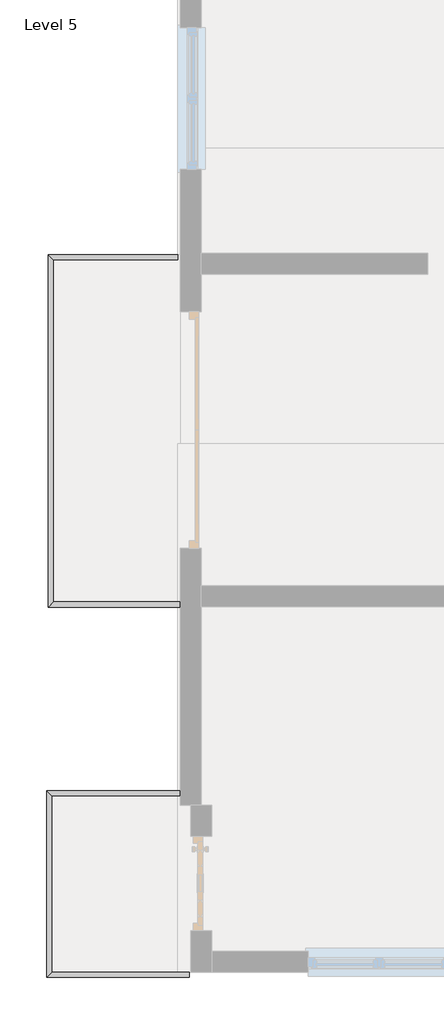
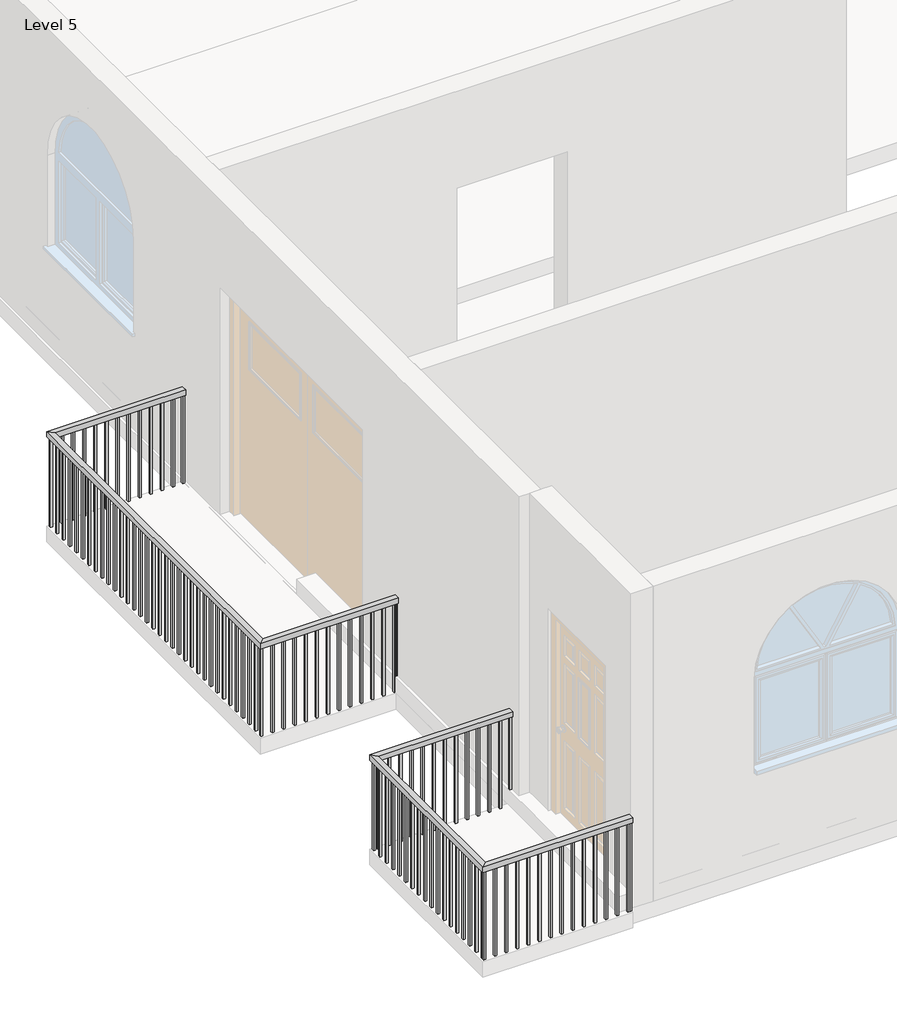
# One storey, part 3 of 7: 2 railings.
"""IFC4 building model written with IfcOpenShell, lengths in millimetres."""

from ifc_helpers import new_model, si_unit, frame, origin, place, context, project, spatial, polyline, outline, extrude, faceted_brep, element, save

model = new_model("IFC4")

# Units and contexts
model_context = context("Model", 3, world=origin())
ifc_project = project(units=[si_unit("LENGTHUNIT", "METRE", prefix="MILLI")], contexts=[model_context])

# Site, building, storey
site = spatial("IfcSite", under=ifc_project)
building = spatial("IfcBuilding", under=site)
storey = spatial("IfcBuildingStorey", under=building, Name="Level 5", Elevation=12192.0)

# Railings
placement = place(None, origin())
element("IfcRailing", 1, ObjectType="Handrail - Rectangular", at=placement, inside=storey, context=model_context, shape_type="SolidModel", body=[
    faceted_brep([(-6354.2109037, -3767.6037749, 13106.4), (-6354.2109037, -3767.6037749, 13055.6), (-6354.2109037, -3716.8037749, 13055.6), (-6354.2109037, -3716.8037749, 13106.4), (-7548.0109037, -3767.6037749, 13106.4), (-7548.0109037, -3767.6037749, 13055.6), (-7598.8109037, -3716.8037749, 13055.6), (-7598.8109037, -3716.8037749, 13106.4), (-7548.0109037, -7054.4894702, 13106.4), (-7548.0109037, -7054.4894702, 13055.6), (-7598.8109037, -7105.2894702, 13055.6), (-7598.8109037, -7105.2894702, 13106.4), (-6330.8013636, -7054.4894702, 13106.4), (-6330.8013636, -7105.2894702, 13106.4), (-6330.8013636, -7105.2894702, 13055.6), (-6330.8013636, -7054.4894702, 13055.6)], [[[0, 1, 2, 3]], [[1, 0, 4, 5]], [[2, 1, 5, 6]], [[3, 2, 6, 7]], [[0, 3, 7, 4]], [[5, 4, 8, 9]], [[6, 5, 9, 10]], [[7, 6, 10, 11]], [[4, 7, 11, 8]], [[12, 13, 14, 15]], [[9, 8, 12, 15]], [[10, 9, 15, 14]], [[11, 10, 14, 13]], [[8, 11, 13, 12]]]),
    extrude(outline(polyline([(-6363.7359037, -7089.4144702), (-6363.7359037, -7070.3644702), (-6344.6859037, -7070.3644702), (-6344.6859037, -7089.4144702), (-6363.7359037, -7089.4144702)])), frame((0.0, 0.0, 12192.0), z_axis=(0.0, 0.0, 1.0), x_axis=(1.0, 0.0, 0.0)), (0.0, 0.0, 1.0), 863.6),
    extrude(outline(polyline([(-6465.3359037, -7089.4144702), (-6465.3359037, -7070.3644702), (-6446.2859037, -7070.3644702), (-6446.2859037, -7089.4144702), (-6465.3359037, -7089.4144702)])), frame((0.0, 0.0, 12192.0), z_axis=(0.0, 0.0, 1.0), x_axis=(1.0, 0.0, 0.0)), (0.0, 0.0, 1.0), 863.6),
    extrude(outline(polyline([(-6566.9359037, -7089.4144702), (-6566.9359037, -7070.3644702), (-6547.8859037, -7070.3644702), (-6547.8859037, -7089.4144702), (-6566.9359037, -7089.4144702)])), frame((0.0, 0.0, 12192.0), z_axis=(0.0, 0.0, 1.0), x_axis=(1.0, 0.0, 0.0)), (0.0, 0.0, 1.0), 863.6),
    extrude(outline(polyline([(-6668.5359037, -7089.4144702), (-6668.5359037, -7070.3644702), (-6649.4859037, -7070.3644702), (-6649.4859037, -7089.4144702), (-6668.5359037, -7089.4144702)])), frame((0.0, 0.0, 12192.0), z_axis=(0.0, 0.0, 1.0), x_axis=(1.0, 0.0, 0.0)), (0.0, 0.0, 1.0), 863.6),
    extrude(outline(polyline([(-6770.1359037, -7089.4144702), (-6770.1359037, -7070.3644702), (-6751.0859037, -7070.3644702), (-6751.0859037, -7089.4144702), (-6770.1359037, -7089.4144702)])), frame((0.0, 0.0, 12192.0), z_axis=(0.0, 0.0, 1.0), x_axis=(1.0, 0.0, 0.0)), (0.0, 0.0, 1.0), 863.6),
    extrude(outline(polyline([(-6871.7359037, -7089.4144702), (-6871.7359037, -7070.3644702), (-6852.6859037, -7070.3644702), (-6852.6859037, -7089.4144702), (-6871.7359037, -7089.4144702)])), frame((0.0, 0.0, 12192.0), z_axis=(0.0, 0.0, 1.0), x_axis=(1.0, 0.0, 0.0)), (0.0, 0.0, 1.0), 863.6),
    extrude(outline(polyline([(-6973.3359037, -7089.4144702), (-6973.3359037, -7070.3644702), (-6954.2859037, -7070.3644702), (-6954.2859037, -7089.4144702), (-6973.3359037, -7089.4144702)])), frame((0.0, 0.0, 12192.0), z_axis=(0.0, 0.0, 1.0), x_axis=(1.0, 0.0, 0.0)), (0.0, 0.0, 1.0), 863.6),
    extrude(outline(polyline([(-7074.9359037, -7089.4144702), (-7074.9359037, -7070.3644702), (-7055.8859037, -7070.3644702), (-7055.8859037, -7089.4144702), (-7074.9359037, -7089.4144702)])), frame((0.0, 0.0, 12192.0), z_axis=(0.0, 0.0, 1.0), x_axis=(1.0, 0.0, 0.0)), (0.0, 0.0, 1.0), 863.6),
    extrude(outline(polyline([(-7176.5359037, -7089.4144702), (-7176.5359037, -7070.3644702), (-7157.4859037, -7070.3644702), (-7157.4859037, -7089.4144702), (-7176.5359037, -7089.4144702)])), frame((0.0, 0.0, 12192.0), z_axis=(0.0, 0.0, 1.0), x_axis=(1.0, 0.0, 0.0)), (0.0, 0.0, 1.0), 863.6),
    extrude(outline(polyline([(-7278.1359037, -7089.4144702), (-7278.1359037, -7070.3644702), (-7259.0859037, -7070.3644702), (-7259.0859037, -7089.4144702), (-7278.1359037, -7089.4144702)])), frame((0.0, 0.0, 12192.0), z_axis=(0.0, 0.0, 1.0), x_axis=(1.0, 0.0, 0.0)), (0.0, 0.0, 1.0), 863.6),
    extrude(outline(polyline([(-7379.7359037, -7089.4144702), (-7379.7359037, -7070.3644702), (-7360.6859037, -7070.3644702), (-7360.6859037, -7089.4144702), (-7379.7359037, -7089.4144702)])), frame((0.0, 0.0, 12192.0), z_axis=(0.0, 0.0, 1.0), x_axis=(1.0, 0.0, 0.0)), (0.0, 0.0, 1.0), 863.6),
    extrude(outline(polyline([(-7481.3359037, -7089.4144702), (-7481.3359037, -7070.3644702), (-7462.2859037, -7070.3644702), (-7462.2859037, -7089.4144702), (-7481.3359037, -7089.4144702)])), frame((0.0, 0.0, 12192.0), z_axis=(0.0, 0.0, 1.0), x_axis=(1.0, 0.0, 0.0)), (0.0, 0.0, 1.0), 863.6),
    extrude(outline(polyline([(-7582.9359037, -6983.8787749), (-7563.8859037, -6983.8787749), (-7563.8859037, -7002.9287749), (-7582.9359037, -7002.9287749), (-7582.9359037, -6983.8787749)])), frame((0.0, 0.0, 12192.0), z_axis=(0.0, 0.0, 1.0), x_axis=(1.0, 0.0, 0.0)), (0.0, 0.0, 1.0), 863.6),
    extrude(outline(polyline([(-7582.9359037, -6882.2787749), (-7563.8859037, -6882.2787749), (-7563.8859037, -6901.3287749), (-7582.9359037, -6901.3287749), (-7582.9359037, -6882.2787749)])), frame((0.0, 0.0, 12192.0), z_axis=(0.0, 0.0, 1.0), x_axis=(1.0, 0.0, 0.0)), (0.0, 0.0, 1.0), 863.6),
    extrude(outline(polyline([(-7582.9359037, -6780.6787749), (-7563.8859037, -6780.6787749), (-7563.8859037, -6799.7287749), (-7582.9359037, -6799.7287749), (-7582.9359037, -6780.6787749)])), frame((0.0, 0.0, 12192.0), z_axis=(0.0, 0.0, 1.0), x_axis=(1.0, 0.0, 0.0)), (0.0, 0.0, 1.0), 863.6),
    extrude(outline(polyline([(-7582.9359037, -6679.0787749), (-7563.8859037, -6679.0787749), (-7563.8859037, -6698.1287749), (-7582.9359037, -6698.1287749), (-7582.9359037, -6679.0787749)])), frame((0.0, 0.0, 12192.0), z_axis=(0.0, 0.0, 1.0), x_axis=(1.0, 0.0, 0.0)), (0.0, 0.0, 1.0), 863.6),
    extrude(outline(polyline([(-7582.9359037, -6577.4787749), (-7563.8859037, -6577.4787749), (-7563.8859037, -6596.5287749), (-7582.9359037, -6596.5287749), (-7582.9359037, -6577.4787749)])), frame((0.0, 0.0, 12192.0), z_axis=(0.0, 0.0, 1.0), x_axis=(1.0, 0.0, 0.0)), (0.0, 0.0, 1.0), 863.6),
    extrude(outline(polyline([(-7582.9359037, -6475.8787749), (-7563.8859037, -6475.8787749), (-7563.8859037, -6494.9287749), (-7582.9359037, -6494.9287749), (-7582.9359037, -6475.8787749)])), frame((0.0, 0.0, 12192.0), z_axis=(0.0, 0.0, 1.0), x_axis=(1.0, 0.0, 0.0)), (0.0, 0.0, 1.0), 863.6),
    extrude(outline(polyline([(-7582.9359037, -6374.2787749), (-7563.8859037, -6374.2787749), (-7563.8859037, -6393.3287749), (-7582.9359037, -6393.3287749), (-7582.9359037, -6374.2787749)])), frame((0.0, 0.0, 12192.0), z_axis=(0.0, 0.0, 1.0), x_axis=(1.0, 0.0, 0.0)), (0.0, 0.0, 1.0), 863.6),
    extrude(outline(polyline([(-7582.9359037, -6272.6787749), (-7563.8859037, -6272.6787749), (-7563.8859037, -6291.7287749), (-7582.9359037, -6291.7287749), (-7582.9359037, -6272.6787749)])), frame((0.0, 0.0, 12192.0), z_axis=(0.0, 0.0, 1.0), x_axis=(1.0, 0.0, 0.0)), (0.0, 0.0, 1.0), 863.6),
    extrude(outline(polyline([(-7582.9359037, -6171.0787749), (-7563.8859037, -6171.0787749), (-7563.8859037, -6190.1287749), (-7582.9359037, -6190.1287749), (-7582.9359037, -6171.0787749)])), frame((0.0, 0.0, 12192.0), z_axis=(0.0, 0.0, 1.0), x_axis=(1.0, 0.0, 0.0)), (0.0, 0.0, 1.0), 863.6),
    extrude(outline(polyline([(-7582.9359037, -6069.4787749), (-7563.8859037, -6069.4787749), (-7563.8859037, -6088.5287749), (-7582.9359037, -6088.5287749), (-7582.9359037, -6069.4787749)])), frame((0.0, 0.0, 12192.0), z_axis=(0.0, 0.0, 1.0), x_axis=(1.0, 0.0, 0.0)), (0.0, 0.0, 1.0), 863.6),
    extrude(outline(polyline([(-7582.9359037, -5967.8787749), (-7563.8859037, -5967.8787749), (-7563.8859037, -5986.9287749), (-7582.9359037, -5986.9287749), (-7582.9359037, -5967.8787749)])), frame((0.0, 0.0, 12192.0), z_axis=(0.0, 0.0, 1.0), x_axis=(1.0, 0.0, 0.0)), (0.0, 0.0, 1.0), 863.6),
    extrude(outline(polyline([(-7582.9359037, -5866.2787749), (-7563.8859037, -5866.2787749), (-7563.8859037, -5885.3287749), (-7582.9359037, -5885.3287749), (-7582.9359037, -5866.2787749)])), frame((0.0, 0.0, 12192.0), z_axis=(0.0, 0.0, 1.0), x_axis=(1.0, 0.0, 0.0)), (0.0, 0.0, 1.0), 863.6),
    extrude(outline(polyline([(-7582.9359037, -5764.6787749), (-7563.8859037, -5764.6787749), (-7563.8859037, -5783.7287749), (-7582.9359037, -5783.7287749), (-7582.9359037, -5764.6787749)])), frame((0.0, 0.0, 12192.0), z_axis=(0.0, 0.0, 1.0), x_axis=(1.0, 0.0, 0.0)), (0.0, 0.0, 1.0), 863.6),
    extrude(outline(polyline([(-7582.9359037, -5663.0787749), (-7563.8859037, -5663.0787749), (-7563.8859037, -5682.1287749), (-7582.9359037, -5682.1287749), (-7582.9359037, -5663.0787749)])), frame((0.0, 0.0, 12192.0), z_axis=(0.0, 0.0, 1.0), x_axis=(1.0, 0.0, 0.0)), (0.0, 0.0, 1.0), 863.6),
    extrude(outline(polyline([(-7582.9359037, -5561.4787749), (-7563.8859037, -5561.4787749), (-7563.8859037, -5580.5287749), (-7582.9359037, -5580.5287749), (-7582.9359037, -5561.4787749)])), frame((0.0, 0.0, 12192.0), z_axis=(0.0, 0.0, 1.0), x_axis=(1.0, 0.0, 0.0)), (0.0, 0.0, 1.0), 863.6),
    extrude(outline(polyline([(-7582.9359037, -5459.8787749), (-7563.8859037, -5459.8787749), (-7563.8859037, -5478.9287749), (-7582.9359037, -5478.9287749), (-7582.9359037, -5459.8787749)])), frame((0.0, 0.0, 12192.0), z_axis=(0.0, 0.0, 1.0), x_axis=(1.0, 0.0, 0.0)), (0.0, 0.0, 1.0), 863.6),
    extrude(outline(polyline([(-7582.9359037, -5358.2787749), (-7563.8859037, -5358.2787749), (-7563.8859037, -5377.3287749), (-7582.9359037, -5377.3287749), (-7582.9359037, -5358.2787749)])), frame((0.0, 0.0, 12192.0), z_axis=(0.0, 0.0, 1.0), x_axis=(1.0, 0.0, 0.0)), (0.0, 0.0, 1.0), 863.6),
    extrude(outline(polyline([(-7582.9359037, -5256.6787749), (-7563.8859037, -5256.6787749), (-7563.8859037, -5275.7287749), (-7582.9359037, -5275.7287749), (-7582.9359037, -5256.6787749)])), frame((0.0, 0.0, 12192.0), z_axis=(0.0, 0.0, 1.0), x_axis=(1.0, 0.0, 0.0)), (0.0, 0.0, 1.0), 863.6),
    extrude(outline(polyline([(-7582.9359037, -5155.0787749), (-7563.8859037, -5155.0787749), (-7563.8859037, -5174.1287749), (-7582.9359037, -5174.1287749), (-7582.9359037, -5155.0787749)])), frame((0.0, 0.0, 12192.0), z_axis=(0.0, 0.0, 1.0), x_axis=(1.0, 0.0, 0.0)), (0.0, 0.0, 1.0), 863.6),
    extrude(outline(polyline([(-7582.9359037, -5053.4787749), (-7563.8859037, -5053.4787749), (-7563.8859037, -5072.5287749), (-7582.9359037, -5072.5287749), (-7582.9359037, -5053.4787749)])), frame((0.0, 0.0, 12192.0), z_axis=(0.0, 0.0, 1.0), x_axis=(1.0, 0.0, 0.0)), (0.0, 0.0, 1.0), 863.6),
    extrude(outline(polyline([(-7582.9359037, -4951.8787749), (-7563.8859037, -4951.8787749), (-7563.8859037, -4970.9287749), (-7582.9359037, -4970.9287749), (-7582.9359037, -4951.8787749)])), frame((0.0, 0.0, 12192.0), z_axis=(0.0, 0.0, 1.0), x_axis=(1.0, 0.0, 0.0)), (0.0, 0.0, 1.0), 863.6),
    extrude(outline(polyline([(-7582.9359037, -4850.2787749), (-7563.8859037, -4850.2787749), (-7563.8859037, -4869.3287749), (-7582.9359037, -4869.3287749), (-7582.9359037, -4850.2787749)])), frame((0.0, 0.0, 12192.0), z_axis=(0.0, 0.0, 1.0), x_axis=(1.0, 0.0, 0.0)), (0.0, 0.0, 1.0), 863.6),
    extrude(outline(polyline([(-7582.9359037, -4748.6787749), (-7563.8859037, -4748.6787749), (-7563.8859037, -4767.7287749), (-7582.9359037, -4767.7287749), (-7582.9359037, -4748.6787749)])), frame((0.0, 0.0, 12192.0), z_axis=(0.0, 0.0, 1.0), x_axis=(1.0, 0.0, 0.0)), (0.0, 0.0, 1.0), 863.6),
    extrude(outline(polyline([(-7582.9359037, -4647.0787749), (-7563.8859037, -4647.0787749), (-7563.8859037, -4666.1287749), (-7582.9359037, -4666.1287749), (-7582.9359037, -4647.0787749)])), frame((0.0, 0.0, 12192.0), z_axis=(0.0, 0.0, 1.0), x_axis=(1.0, 0.0, 0.0)), (0.0, 0.0, 1.0), 863.6),
    extrude(outline(polyline([(-7582.9359037, -4545.4787749), (-7563.8859037, -4545.4787749), (-7563.8859037, -4564.5287749), (-7582.9359037, -4564.5287749), (-7582.9359037, -4545.4787749)])), frame((0.0, 0.0, 12192.0), z_axis=(0.0, 0.0, 1.0), x_axis=(1.0, 0.0, 0.0)), (0.0, 0.0, 1.0), 863.6),
    extrude(outline(polyline([(-7582.9359037, -4443.8787749), (-7563.8859037, -4443.8787749), (-7563.8859037, -4462.9287749), (-7582.9359037, -4462.9287749), (-7582.9359037, -4443.8787749)])), frame((0.0, 0.0, 12192.0), z_axis=(0.0, 0.0, 1.0), x_axis=(1.0, 0.0, 0.0)), (0.0, 0.0, 1.0), 863.6),
    extrude(outline(polyline([(-7582.9359037, -4342.2787749), (-7563.8859037, -4342.2787749), (-7563.8859037, -4361.3287749), (-7582.9359037, -4361.3287749), (-7582.9359037, -4342.2787749)])), frame((0.0, 0.0, 12192.0), z_axis=(0.0, 0.0, 1.0), x_axis=(1.0, 0.0, 0.0)), (0.0, 0.0, 1.0), 863.6),
    extrude(outline(polyline([(-7582.9359037, -4240.6787749), (-7563.8859037, -4240.6787749), (-7563.8859037, -4259.7287749), (-7582.9359037, -4259.7287749), (-7582.9359037, -4240.6787749)])), frame((0.0, 0.0, 12192.0), z_axis=(0.0, 0.0, 1.0), x_axis=(1.0, 0.0, 0.0)), (0.0, 0.0, 1.0), 863.6),
    extrude(outline(polyline([(-7582.9359037, -4139.0787749), (-7563.8859037, -4139.0787749), (-7563.8859037, -4158.1287749), (-7582.9359037, -4158.1287749), (-7582.9359037, -4139.0787749)])), frame((0.0, 0.0, 12192.0), z_axis=(0.0, 0.0, 1.0), x_axis=(1.0, 0.0, 0.0)), (0.0, 0.0, 1.0), 863.6),
    extrude(outline(polyline([(-7582.9359037, -4037.4787749), (-7563.8859037, -4037.4787749), (-7563.8859037, -4056.5287749), (-7582.9359037, -4056.5287749), (-7582.9359037, -4037.4787749)])), frame((0.0, 0.0, 12192.0), z_axis=(0.0, 0.0, 1.0), x_axis=(1.0, 0.0, 0.0)), (0.0, 0.0, 1.0), 863.6),
    extrude(outline(polyline([(-7582.9359037, -3935.8787749), (-7563.8859037, -3935.8787749), (-7563.8859037, -3954.9287749), (-7582.9359037, -3954.9287749), (-7582.9359037, -3935.8787749)])), frame((0.0, 0.0, 12192.0), z_axis=(0.0, 0.0, 1.0), x_axis=(1.0, 0.0, 0.0)), (0.0, 0.0, 1.0), 863.6),
    extrude(outline(polyline([(-7582.9359037, -3834.2787749), (-7563.8859037, -3834.2787749), (-7563.8859037, -3853.3287749), (-7582.9359037, -3853.3287749), (-7582.9359037, -3834.2787749)])), frame((0.0, 0.0, 12192.0), z_axis=(0.0, 0.0, 1.0), x_axis=(1.0, 0.0, 0.0)), (0.0, 0.0, 1.0), 863.6),
    extrude(outline(polyline([(-7462.2859037, -3732.6787749), (-7462.2859037, -3751.7287749), (-7481.3359037, -3751.7287749), (-7481.3359037, -3732.6787749), (-7462.2859037, -3732.6787749)])), frame((0.0, 0.0, 12192.0), z_axis=(0.0, 0.0, 1.0), x_axis=(1.0, 0.0, 0.0)), (0.0, 0.0, 1.0), 863.6),
    extrude(outline(polyline([(-7360.6859037, -3732.6787749), (-7360.6859037, -3751.7287749), (-7379.7359037, -3751.7287749), (-7379.7359037, -3732.6787749), (-7360.6859037, -3732.6787749)])), frame((0.0, 0.0, 12192.0), z_axis=(0.0, 0.0, 1.0), x_axis=(1.0, 0.0, 0.0)), (0.0, 0.0, 1.0), 863.6),
    extrude(outline(polyline([(-7259.0859037, -3732.6787749), (-7259.0859037, -3751.7287749), (-7278.1359037, -3751.7287749), (-7278.1359037, -3732.6787749), (-7259.0859037, -3732.6787749)])), frame((0.0, 0.0, 12192.0), z_axis=(0.0, 0.0, 1.0), x_axis=(1.0, 0.0, 0.0)), (0.0, 0.0, 1.0), 863.6),
    extrude(outline(polyline([(-7157.4859037, -3732.6787749), (-7157.4859037, -3751.7287749), (-7176.5359037, -3751.7287749), (-7176.5359037, -3732.6787749), (-7157.4859037, -3732.6787749)])), frame((0.0, 0.0, 12192.0), z_axis=(0.0, 0.0, 1.0), x_axis=(1.0, 0.0, 0.0)), (0.0, 0.0, 1.0), 863.6),
    extrude(outline(polyline([(-7055.8859037, -3732.6787749), (-7055.8859037, -3751.7287749), (-7074.9359037, -3751.7287749), (-7074.9359037, -3732.6787749), (-7055.8859037, -3732.6787749)])), frame((0.0, 0.0, 12192.0), z_axis=(0.0, 0.0, 1.0), x_axis=(1.0, 0.0, 0.0)), (0.0, 0.0, 1.0), 863.6),
    extrude(outline(polyline([(-6954.2859037, -3732.6787749), (-6954.2859037, -3751.7287749), (-6973.3359037, -3751.7287749), (-6973.3359037, -3732.6787749), (-6954.2859037, -3732.6787749)])), frame((0.0, 0.0, 12192.0), z_axis=(0.0, 0.0, 1.0), x_axis=(1.0, 0.0, 0.0)), (0.0, 0.0, 1.0), 863.6),
    extrude(outline(polyline([(-6852.6859037, -3732.6787749), (-6852.6859037, -3751.7287749), (-6871.7359037, -3751.7287749), (-6871.7359037, -3732.6787749), (-6852.6859037, -3732.6787749)])), frame((0.0, 0.0, 12192.0), z_axis=(0.0, 0.0, 1.0), x_axis=(1.0, 0.0, 0.0)), (0.0, 0.0, 1.0), 863.6),
    extrude(outline(polyline([(-6751.0859037, -3732.6787749), (-6751.0859037, -3751.7287749), (-6770.1359037, -3751.7287749), (-6770.1359037, -3732.6787749), (-6751.0859037, -3732.6787749)])), frame((0.0, 0.0, 12192.0), z_axis=(0.0, 0.0, 1.0), x_axis=(1.0, 0.0, 0.0)), (0.0, 0.0, 1.0), 863.6),
    extrude(outline(polyline([(-6649.4859037, -3732.6787749), (-6649.4859037, -3751.7287749), (-6668.5359037, -3751.7287749), (-6668.5359037, -3732.6787749), (-6649.4859037, -3732.6787749)])), frame((0.0, 0.0, 12192.0), z_axis=(0.0, 0.0, 1.0), x_axis=(1.0, 0.0, 0.0)), (0.0, 0.0, 1.0), 863.6),
    extrude(outline(polyline([(-6547.8859037, -3732.6787749), (-6547.8859037, -3751.7287749), (-6566.9359037, -3751.7287749), (-6566.9359037, -3732.6787749), (-6547.8859037, -3732.6787749)])), frame((0.0, 0.0, 12192.0), z_axis=(0.0, 0.0, 1.0), x_axis=(1.0, 0.0, 0.0)), (0.0, 0.0, 1.0), 863.6),
    extrude(outline(polyline([(-6446.2859037, -3732.6787749), (-6446.2859037, -3751.7287749), (-6465.3359037, -3751.7287749), (-6465.3359037, -3732.6787749), (-6446.2859037, -3732.6787749)])), frame((0.0, 0.0, 12192.0), z_axis=(0.0, 0.0, 1.0), x_axis=(1.0, 0.0, 0.0)), (0.0, 0.0, 1.0), 863.6),
    extrude(outline(polyline([(-7582.9359037, -7070.3644702), (-7563.8859037, -7070.3644702), (-7563.8859037, -7089.4144702), (-7582.9359037, -7089.4144702), (-7582.9359037, -7070.3644702)])), frame((0.0, 0.0, 12192.0), z_axis=(0.0, 0.0, 1.0), x_axis=(1.0, 0.0, 0.0)), (0.0, 0.0, 1.0), 863.6),
    extrude(outline(polyline([(-7563.8859037, -3732.6787749), (-7563.8859037, -3751.7287749), (-7582.9359037, -3751.7287749), (-7582.9359037, -3732.6787749), (-7563.8859037, -3732.6787749)])), frame((0.0, 0.0, 12192.0), z_axis=(0.0, 0.0, 1.0), x_axis=(1.0, 0.0, 0.0)), (0.0, 0.0, 1.0), 863.6),
    extrude(outline(polyline([(-6349.8513636, -7089.4144702), (-6349.8513636, -7070.3644702), (-6330.8013636, -7070.3644702), (-6330.8013636, -7089.4144702), (-6349.8513636, -7089.4144702)])), frame((0.0, 0.0, 12192.0), z_axis=(0.0, 0.0, 1.0), x_axis=(1.0, 0.0, 0.0)), (0.0, 0.0, 1.0), 863.6),
    extrude(outline(polyline([(-6354.2109037, -3732.6787749), (-6354.2109037, -3751.7287749), (-6373.2609037, -3751.7287749), (-6373.2609037, -3732.6787749), (-6354.2109037, -3732.6787749)])), frame((0.0, 0.0, 12192.0), z_axis=(0.0, 0.0, 1.0), x_axis=(1.0, 0.0, 0.0)), (0.0, 0.0, 1.0), 863.6),
])
element("IfcRailing", 2, ObjectType="Handrail - Rectangular", at=placement, inside=storey, context=model_context, shape_type="SolidModel", body=[
    faceted_brep([(-6330.8013636, -8918.8845215, 13106.4), (-6330.8013636, -8918.8845215, 13055.6), (-6330.8013636, -8868.0845215, 13055.6), (-6330.8013636, -8868.0845215, 13106.4), (-7563.8859037, -8918.8845215, 13106.4), (-7563.8859037, -8918.8845215, 13055.6), (-7614.6859037, -8868.0845215, 13055.6), (-7614.6859037, -8868.0845215, 13106.4), (-7563.8859037, -10612.9037749, 13106.4), (-7563.8859037, -10612.9037749, 13055.6), (-7614.6859037, -10663.7037749, 13055.6), (-7614.6859037, -10663.7037749, 13106.4), (-6243.0859037, -10612.9037749, 13106.4), (-6243.0859037, -10663.7037749, 13106.4), (-6243.0859037, -10663.7037749, 13055.6), (-6243.0859037, -10612.9037749, 13055.6)], [[[0, 1, 2, 3]], [[1, 0, 4, 5]], [[2, 1, 5, 6]], [[3, 2, 6, 7]], [[0, 3, 7, 4]], [[5, 4, 8, 9]], [[6, 5, 9, 10]], [[7, 6, 10, 11]], [[4, 7, 11, 8]], [[12, 13, 14, 15]], [[9, 8, 12, 15]], [[10, 9, 15, 14]], [[11, 10, 14, 13]], [[8, 11, 13, 12]]]),
    extrude(outline(polyline([(-6278.0109037, -10647.8287749), (-6278.0109037, -10628.7787749), (-6258.9609037, -10628.7787749), (-6258.9609037, -10647.8287749), (-6278.0109037, -10647.8287749)])), frame((0.0, 0.0, 12192.0), z_axis=(0.0, 0.0, 1.0), x_axis=(1.0, 0.0, 0.0)), (0.0, 0.0, 1.0), 863.6),
    extrude(outline(polyline([(-6379.6109037, -10647.8287749), (-6379.6109037, -10628.7787749), (-6360.5609037, -10628.7787749), (-6360.5609037, -10647.8287749), (-6379.6109037, -10647.8287749)])), frame((0.0, 0.0, 12192.0), z_axis=(0.0, 0.0, 1.0), x_axis=(1.0, 0.0, 0.0)), (0.0, 0.0, 1.0), 863.6),
    extrude(outline(polyline([(-6481.2109037, -10647.8287749), (-6481.2109037, -10628.7787749), (-6462.1609037, -10628.7787749), (-6462.1609037, -10647.8287749), (-6481.2109037, -10647.8287749)])), frame((0.0, 0.0, 12192.0), z_axis=(0.0, 0.0, 1.0), x_axis=(1.0, 0.0, 0.0)), (0.0, 0.0, 1.0), 863.6),
    extrude(outline(polyline([(-6582.8109037, -10647.8287749), (-6582.8109037, -10628.7787749), (-6563.7609037, -10628.7787749), (-6563.7609037, -10647.8287749), (-6582.8109037, -10647.8287749)])), frame((0.0, 0.0, 12192.0), z_axis=(0.0, 0.0, 1.0), x_axis=(1.0, 0.0, 0.0)), (0.0, 0.0, 1.0), 863.6),
    extrude(outline(polyline([(-6684.4109037, -10647.8287749), (-6684.4109037, -10628.7787749), (-6665.3609037, -10628.7787749), (-6665.3609037, -10647.8287749), (-6684.4109037, -10647.8287749)])), frame((0.0, 0.0, 12192.0), z_axis=(0.0, 0.0, 1.0), x_axis=(1.0, 0.0, 0.0)), (0.0, 0.0, 1.0), 863.6),
    extrude(outline(polyline([(-6786.0109037, -10647.8287749), (-6786.0109037, -10628.7787749), (-6766.9609037, -10628.7787749), (-6766.9609037, -10647.8287749), (-6786.0109037, -10647.8287749)])), frame((0.0, 0.0, 12192.0), z_axis=(0.0, 0.0, 1.0), x_axis=(1.0, 0.0, 0.0)), (0.0, 0.0, 1.0), 863.6),
    extrude(outline(polyline([(-6887.6109037, -10647.8287749), (-6887.6109037, -10628.7787749), (-6868.5609037, -10628.7787749), (-6868.5609037, -10647.8287749), (-6887.6109037, -10647.8287749)])), frame((0.0, 0.0, 12192.0), z_axis=(0.0, 0.0, 1.0), x_axis=(1.0, 0.0, 0.0)), (0.0, 0.0, 1.0), 863.6),
    extrude(outline(polyline([(-6989.2109037, -10647.8287749), (-6989.2109037, -10628.7787749), (-6970.1609037, -10628.7787749), (-6970.1609037, -10647.8287749), (-6989.2109037, -10647.8287749)])), frame((0.0, 0.0, 12192.0), z_axis=(0.0, 0.0, 1.0), x_axis=(1.0, 0.0, 0.0)), (0.0, 0.0, 1.0), 863.6),
    extrude(outline(polyline([(-7090.8109037, -10647.8287749), (-7090.8109037, -10628.7787749), (-7071.7609037, -10628.7787749), (-7071.7609037, -10647.8287749), (-7090.8109037, -10647.8287749)])), frame((0.0, 0.0, 12192.0), z_axis=(0.0, 0.0, 1.0), x_axis=(1.0, 0.0, 0.0)), (0.0, 0.0, 1.0), 863.6),
    extrude(outline(polyline([(-7192.4109037, -10647.8287749), (-7192.4109037, -10628.7787749), (-7173.3609037, -10628.7787749), (-7173.3609037, -10647.8287749), (-7192.4109037, -10647.8287749)])), frame((0.0, 0.0, 12192.0), z_axis=(0.0, 0.0, 1.0), x_axis=(1.0, 0.0, 0.0)), (0.0, 0.0, 1.0), 863.6),
    extrude(outline(polyline([(-7294.0109037, -10647.8287749), (-7294.0109037, -10628.7787749), (-7274.9609037, -10628.7787749), (-7274.9609037, -10647.8287749), (-7294.0109037, -10647.8287749)])), frame((0.0, 0.0, 12192.0), z_axis=(0.0, 0.0, 1.0), x_axis=(1.0, 0.0, 0.0)), (0.0, 0.0, 1.0), 863.6),
    extrude(outline(polyline([(-7395.6109037, -10647.8287749), (-7395.6109037, -10628.7787749), (-7376.5609037, -10628.7787749), (-7376.5609037, -10647.8287749), (-7395.6109037, -10647.8287749)])), frame((0.0, 0.0, 12192.0), z_axis=(0.0, 0.0, 1.0), x_axis=(1.0, 0.0, 0.0)), (0.0, 0.0, 1.0), 863.6),
    extrude(outline(polyline([(-7497.2109037, -10647.8287749), (-7497.2109037, -10628.7787749), (-7478.1609037, -10628.7787749), (-7478.1609037, -10647.8287749), (-7497.2109037, -10647.8287749)])), frame((0.0, 0.0, 12192.0), z_axis=(0.0, 0.0, 1.0), x_axis=(1.0, 0.0, 0.0)), (0.0, 0.0, 1.0), 863.6),
    extrude(outline(polyline([(-7598.8109037, -10611.1595215), (-7579.7609037, -10611.1595215), (-7579.7609037, -10630.2095215), (-7598.8109037, -10630.2095215), (-7598.8109037, -10611.1595215)])), frame((0.0, 0.0, 12192.0), z_axis=(0.0, 0.0, 1.0), x_axis=(1.0, 0.0, 0.0)), (0.0, 0.0, 1.0), 863.6),
    extrude(outline(polyline([(-7598.8109037, -10509.5595215), (-7579.7609037, -10509.5595215), (-7579.7609037, -10528.6095215), (-7598.8109037, -10528.6095215), (-7598.8109037, -10509.5595215)])), frame((0.0, 0.0, 12192.0), z_axis=(0.0, 0.0, 1.0), x_axis=(1.0, 0.0, 0.0)), (0.0, 0.0, 1.0), 863.6),
    extrude(outline(polyline([(-7598.8109037, -10407.9595215), (-7579.7609037, -10407.9595215), (-7579.7609037, -10427.0095215), (-7598.8109037, -10427.0095215), (-7598.8109037, -10407.9595215)])), frame((0.0, 0.0, 12192.0), z_axis=(0.0, 0.0, 1.0), x_axis=(1.0, 0.0, 0.0)), (0.0, 0.0, 1.0), 863.6),
    extrude(outline(polyline([(-7598.8109037, -10306.3595215), (-7579.7609037, -10306.3595215), (-7579.7609037, -10325.4095215), (-7598.8109037, -10325.4095215), (-7598.8109037, -10306.3595215)])), frame((0.0, 0.0, 12192.0), z_axis=(0.0, 0.0, 1.0), x_axis=(1.0, 0.0, 0.0)), (0.0, 0.0, 1.0), 863.6),
    extrude(outline(polyline([(-7598.8109037, -10204.7595215), (-7579.7609037, -10204.7595215), (-7579.7609037, -10223.8095215), (-7598.8109037, -10223.8095215), (-7598.8109037, -10204.7595215)])), frame((0.0, 0.0, 12192.0), z_axis=(0.0, 0.0, 1.0), x_axis=(1.0, 0.0, 0.0)), (0.0, 0.0, 1.0), 863.6),
    extrude(outline(polyline([(-7598.8109037, -10103.1595215), (-7579.7609037, -10103.1595215), (-7579.7609037, -10122.2095215), (-7598.8109037, -10122.2095215), (-7598.8109037, -10103.1595215)])), frame((0.0, 0.0, 12192.0), z_axis=(0.0, 0.0, 1.0), x_axis=(1.0, 0.0, 0.0)), (0.0, 0.0, 1.0), 863.6),
    extrude(outline(polyline([(-7598.8109037, -10001.5595215), (-7579.7609037, -10001.5595215), (-7579.7609037, -10020.6095215), (-7598.8109037, -10020.6095215), (-7598.8109037, -10001.5595215)])), frame((0.0, 0.0, 12192.0), z_axis=(0.0, 0.0, 1.0), x_axis=(1.0, 0.0, 0.0)), (0.0, 0.0, 1.0), 863.6),
    extrude(outline(polyline([(-7598.8109037, -9899.9595215), (-7579.7609037, -9899.9595215), (-7579.7609037, -9919.0095215), (-7598.8109037, -9919.0095215), (-7598.8109037, -9899.9595215)])), frame((0.0, 0.0, 12192.0), z_axis=(0.0, 0.0, 1.0), x_axis=(1.0, 0.0, 0.0)), (0.0, 0.0, 1.0), 863.6),
    extrude(outline(polyline([(-7598.8109037, -9798.3595215), (-7579.7609037, -9798.3595215), (-7579.7609037, -9817.4095215), (-7598.8109037, -9817.4095215), (-7598.8109037, -9798.3595215)])), frame((0.0, 0.0, 12192.0), z_axis=(0.0, 0.0, 1.0), x_axis=(1.0, 0.0, 0.0)), (0.0, 0.0, 1.0), 863.6),
    extrude(outline(polyline([(-7598.8109037, -9696.7595215), (-7579.7609037, -9696.7595215), (-7579.7609037, -9715.8095215), (-7598.8109037, -9715.8095215), (-7598.8109037, -9696.7595215)])), frame((0.0, 0.0, 12192.0), z_axis=(0.0, 0.0, 1.0), x_axis=(1.0, 0.0, 0.0)), (0.0, 0.0, 1.0), 863.6),
    extrude(outline(polyline([(-7598.8109037, -9595.1595215), (-7579.7609037, -9595.1595215), (-7579.7609037, -9614.2095215), (-7598.8109037, -9614.2095215), (-7598.8109037, -9595.1595215)])), frame((0.0, 0.0, 12192.0), z_axis=(0.0, 0.0, 1.0), x_axis=(1.0, 0.0, 0.0)), (0.0, 0.0, 1.0), 863.6),
    extrude(outline(polyline([(-7598.8109037, -9493.5595215), (-7579.7609037, -9493.5595215), (-7579.7609037, -9512.6095215), (-7598.8109037, -9512.6095215), (-7598.8109037, -9493.5595215)])), frame((0.0, 0.0, 12192.0), z_axis=(0.0, 0.0, 1.0), x_axis=(1.0, 0.0, 0.0)), (0.0, 0.0, 1.0), 863.6),
    extrude(outline(polyline([(-7598.8109037, -9391.9595215), (-7579.7609037, -9391.9595215), (-7579.7609037, -9411.0095215), (-7598.8109037, -9411.0095215), (-7598.8109037, -9391.9595215)])), frame((0.0, 0.0, 12192.0), z_axis=(0.0, 0.0, 1.0), x_axis=(1.0, 0.0, 0.0)), (0.0, 0.0, 1.0), 863.6),
    extrude(outline(polyline([(-7598.8109037, -9290.3595215), (-7579.7609037, -9290.3595215), (-7579.7609037, -9309.4095215), (-7598.8109037, -9309.4095215), (-7598.8109037, -9290.3595215)])), frame((0.0, 0.0, 12192.0), z_axis=(0.0, 0.0, 1.0), x_axis=(1.0, 0.0, 0.0)), (0.0, 0.0, 1.0), 863.6),
    extrude(outline(polyline([(-7598.8109037, -9188.7595215), (-7579.7609037, -9188.7595215), (-7579.7609037, -9207.8095215), (-7598.8109037, -9207.8095215), (-7598.8109037, -9188.7595215)])), frame((0.0, 0.0, 12192.0), z_axis=(0.0, 0.0, 1.0), x_axis=(1.0, 0.0, 0.0)), (0.0, 0.0, 1.0), 863.6),
    extrude(outline(polyline([(-7598.8109037, -9087.1595215), (-7579.7609037, -9087.1595215), (-7579.7609037, -9106.2095215), (-7598.8109037, -9106.2095215), (-7598.8109037, -9087.1595215)])), frame((0.0, 0.0, 12192.0), z_axis=(0.0, 0.0, 1.0), x_axis=(1.0, 0.0, 0.0)), (0.0, 0.0, 1.0), 863.6),
    extrude(outline(polyline([(-7598.8109037, -8985.5595215), (-7579.7609037, -8985.5595215), (-7579.7609037, -9004.6095215), (-7598.8109037, -9004.6095215), (-7598.8109037, -8985.5595215)])), frame((0.0, 0.0, 12192.0), z_axis=(0.0, 0.0, 1.0), x_axis=(1.0, 0.0, 0.0)), (0.0, 0.0, 1.0), 863.6),
    extrude(outline(polyline([(-7540.4763636, -8883.9595215), (-7540.4763636, -8903.0095215), (-7559.5263636, -8903.0095215), (-7559.5263636, -8883.9595215), (-7540.4763636, -8883.9595215)])), frame((0.0, 0.0, 12192.0), z_axis=(0.0, 0.0, 1.0), x_axis=(1.0, 0.0, 0.0)), (0.0, 0.0, 1.0), 863.6),
    extrude(outline(polyline([(-7438.8763636, -8883.9595215), (-7438.8763636, -8903.0095215), (-7457.9263636, -8903.0095215), (-7457.9263636, -8883.9595215), (-7438.8763636, -8883.9595215)])), frame((0.0, 0.0, 12192.0), z_axis=(0.0, 0.0, 1.0), x_axis=(1.0, 0.0, 0.0)), (0.0, 0.0, 1.0), 863.6),
    extrude(outline(polyline([(-7337.2763636, -8883.9595215), (-7337.2763636, -8903.0095215), (-7356.3263636, -8903.0095215), (-7356.3263636, -8883.9595215), (-7337.2763636, -8883.9595215)])), frame((0.0, 0.0, 12192.0), z_axis=(0.0, 0.0, 1.0), x_axis=(1.0, 0.0, 0.0)), (0.0, 0.0, 1.0), 863.6),
    extrude(outline(polyline([(-7235.6763636, -8883.9595215), (-7235.6763636, -8903.0095215), (-7254.7263636, -8903.0095215), (-7254.7263636, -8883.9595215), (-7235.6763636, -8883.9595215)])), frame((0.0, 0.0, 12192.0), z_axis=(0.0, 0.0, 1.0), x_axis=(1.0, 0.0, 0.0)), (0.0, 0.0, 1.0), 863.6),
    extrude(outline(polyline([(-7134.0763636, -8883.9595215), (-7134.0763636, -8903.0095215), (-7153.1263636, -8903.0095215), (-7153.1263636, -8883.9595215), (-7134.0763636, -8883.9595215)])), frame((0.0, 0.0, 12192.0), z_axis=(0.0, 0.0, 1.0), x_axis=(1.0, 0.0, 0.0)), (0.0, 0.0, 1.0), 863.6),
    extrude(outline(polyline([(-7032.4763636, -8883.9595215), (-7032.4763636, -8903.0095215), (-7051.5263636, -8903.0095215), (-7051.5263636, -8883.9595215), (-7032.4763636, -8883.9595215)])), frame((0.0, 0.0, 12192.0), z_axis=(0.0, 0.0, 1.0), x_axis=(1.0, 0.0, 0.0)), (0.0, 0.0, 1.0), 863.6),
    extrude(outline(polyline([(-6930.8763636, -8883.9595215), (-6930.8763636, -8903.0095215), (-6949.9263636, -8903.0095215), (-6949.9263636, -8883.9595215), (-6930.8763636, -8883.9595215)])), frame((0.0, 0.0, 12192.0), z_axis=(0.0, 0.0, 1.0), x_axis=(1.0, 0.0, 0.0)), (0.0, 0.0, 1.0), 863.6),
    extrude(outline(polyline([(-6829.2763636, -8883.9595215), (-6829.2763636, -8903.0095215), (-6848.3263636, -8903.0095215), (-6848.3263636, -8883.9595215), (-6829.2763636, -8883.9595215)])), frame((0.0, 0.0, 12192.0), z_axis=(0.0, 0.0, 1.0), x_axis=(1.0, 0.0, 0.0)), (0.0, 0.0, 1.0), 863.6),
    extrude(outline(polyline([(-6727.6763636, -8883.9595215), (-6727.6763636, -8903.0095215), (-6746.7263636, -8903.0095215), (-6746.7263636, -8883.9595215), (-6727.6763636, -8883.9595215)])), frame((0.0, 0.0, 12192.0), z_axis=(0.0, 0.0, 1.0), x_axis=(1.0, 0.0, 0.0)), (0.0, 0.0, 1.0), 863.6),
    extrude(outline(polyline([(-6626.0763636, -8883.9595215), (-6626.0763636, -8903.0095215), (-6645.1263636, -8903.0095215), (-6645.1263636, -8883.9595215), (-6626.0763636, -8883.9595215)])), frame((0.0, 0.0, 12192.0), z_axis=(0.0, 0.0, 1.0), x_axis=(1.0, 0.0, 0.0)), (0.0, 0.0, 1.0), 863.6),
    extrude(outline(polyline([(-6524.4763636, -8883.9595215), (-6524.4763636, -8903.0095215), (-6543.5263636, -8903.0095215), (-6543.5263636, -8883.9595215), (-6524.4763636, -8883.9595215)])), frame((0.0, 0.0, 12192.0), z_axis=(0.0, 0.0, 1.0), x_axis=(1.0, 0.0, 0.0)), (0.0, 0.0, 1.0), 863.6),
    extrude(outline(polyline([(-6422.8763636, -8883.9595215), (-6422.8763636, -8903.0095215), (-6441.9263636, -8903.0095215), (-6441.9263636, -8883.9595215), (-6422.8763636, -8883.9595215)])), frame((0.0, 0.0, 12192.0), z_axis=(0.0, 0.0, 1.0), x_axis=(1.0, 0.0, 0.0)), (0.0, 0.0, 1.0), 863.6),
    extrude(outline(polyline([(-7598.8109037, -10628.7787749), (-7579.7609037, -10628.7787749), (-7579.7609037, -10647.8287749), (-7598.8109037, -10647.8287749), (-7598.8109037, -10628.7787749)])), frame((0.0, 0.0, 12192.0), z_axis=(0.0, 0.0, 1.0), x_axis=(1.0, 0.0, 0.0)), (0.0, 0.0, 1.0), 863.6),
    extrude(outline(polyline([(-7579.7609037, -8883.9595215), (-7579.7609037, -8903.0095215), (-7598.8109037, -8903.0095215), (-7598.8109037, -8883.9595215), (-7579.7609037, -8883.9595215)])), frame((0.0, 0.0, 12192.0), z_axis=(0.0, 0.0, 1.0), x_axis=(1.0, 0.0, 0.0)), (0.0, 0.0, 1.0), 863.6),
    extrude(outline(polyline([(-6262.1359037, -10647.8287749), (-6262.1359037, -10628.7787749), (-6243.0859037, -10628.7787749), (-6243.0859037, -10647.8287749), (-6262.1359037, -10647.8287749)])), frame((0.0, 0.0, 12192.0), z_axis=(0.0, 0.0, 1.0), x_axis=(1.0, 0.0, 0.0)), (0.0, 0.0, 1.0), 863.6),
    extrude(outline(polyline([(-6330.8013636, -8883.9595215), (-6330.8013636, -8903.0095215), (-6349.8513636, -8903.0095215), (-6349.8513636, -8883.9595215), (-6330.8013636, -8883.9595215)])), frame((0.0, 0.0, 12192.0), z_axis=(0.0, 0.0, 1.0), x_axis=(1.0, 0.0, 0.0)), (0.0, 0.0, 1.0), 863.6),
])

save(model, "model.ifc")

# Revit data of these elements
# Type "Handrail - Rectangular"
#   Assembly Code = "C2010400"
#   built-in parameter 1008612 = 0.0416667 (stored number, unit not read)
#   built-in parameter 1008611 = 0.0416667 (stored number, unit not read)
#   built-in parameter 1008609 = 0.333333 (stored number, unit not read)
#   built-in parameter 1008604 = 0.166667 (stored number, unit not read)
#   built-in parameter 1008603 = 0.166667 (stored number, unit not read)
#   Railing Height = 3' - 0"
#   built-in parameter 1008630 = 2
#   built-in parameter 1008610 = 2
#   built-in parameter 1008618 = Baluster - Square : 3/4"
# Elements 1, 2 (IfcRailing, "Handrail - Rectangular")
#   Phase Created = New Construction
